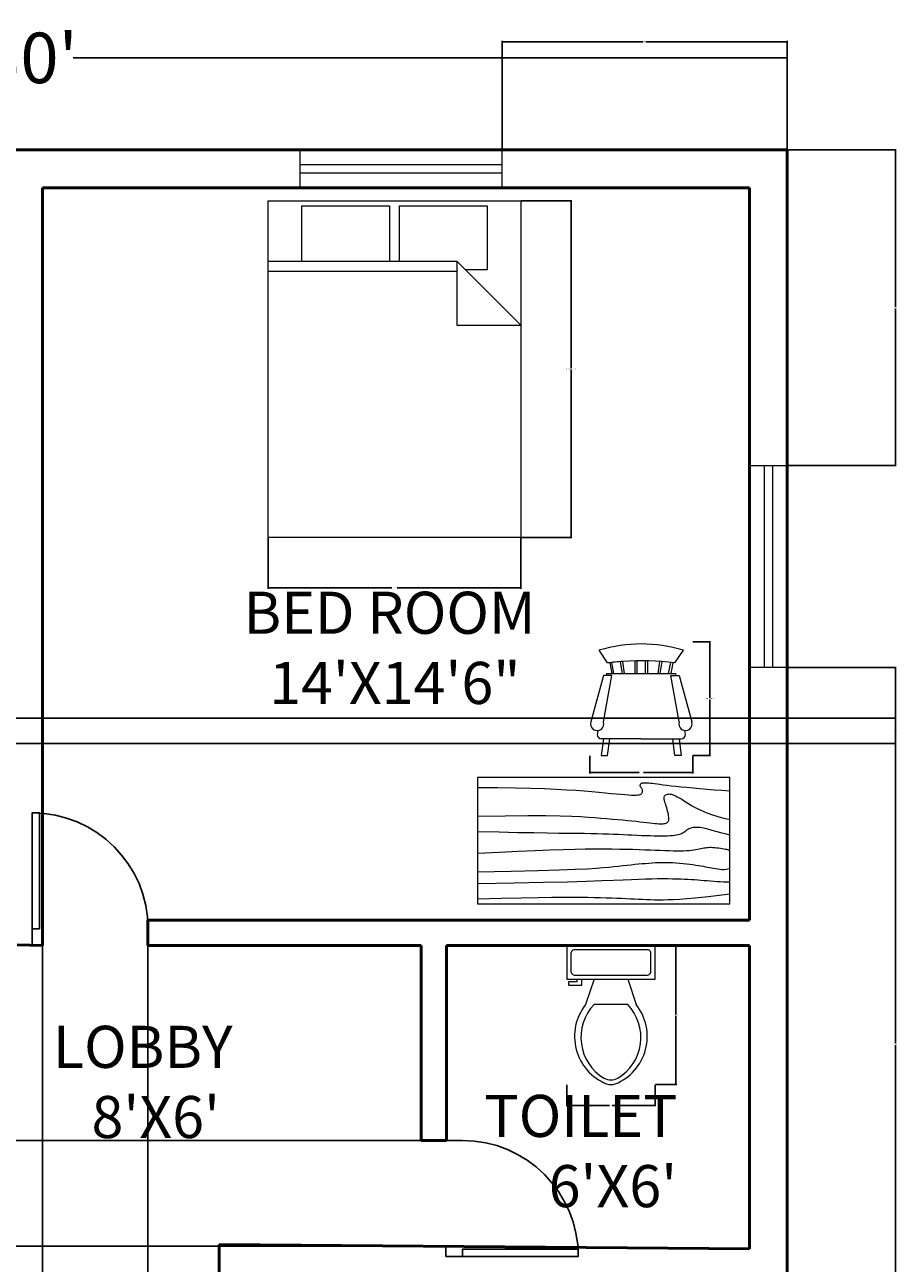
# Model space of a CAD drawing. Units: inches. Extents: x 471 to 898, y -3 to 533.
# Tile 3 of 3: x 691 to 898, y 239 to 533. Entities that reach past the tile are written whole.
import ezdxf

# ---------------------------------------------------------------- set-up
doc = ezdxf.new("R2010")
doc.units = ezdxf.units.IN
doc.header["$MEASUREMENT"] = 0
for name, color, linetype, lineweight in [('A-ANNO-DIMS', 2, 'Continuous', 18), ('A-AREA-IDEN', 7, 'Continuous', 25), ('A-DOOR', 3, 'Continuous', 25), ('A-FLOR-FIXT', 9, 'Continuous', 18), ('A-FURN', 8, 'Continuous', 18), ('A-GLAZ', 4, 'Continuous', 18), ('A-WALL', 7, 'Continuous', 50)]:
    doc.layers.add(name, color=color, linetype=linetype, lineweight=lineweight)
doc.styles.get("Standard").update_dxf_attribs({"font": 'arial.ttf'})
doc.dimstyles.get("Standard").update_dxf_attribs({"dimtxt": 0.18, "dimasz": 0.18, "dimexe": 0.18, "dimexo": 0.0625, "dimgap": 0.09, "dimtad": 0, "dimtih": 1, "dimtoh": 1, "dimdec": 1, "dimzin": 0, "dimdsep": 46, "dimlunit": 4, "dimtxsty": 'Standard', "dimcen": 0.09, "dimadec": 0, "dimazin": 0, "dimtfac": 1, "dimtdec": 1, "dimtofl": 0, "dimtmove": 0, "dimatfit": 3, "dimfxl": 1, "dimtolj": 1, "dimtzin": 0, "dimarcsym": 0})

# ---------------------------------------------------------------- blocks, each defined once
blk = doc.blocks.new('Bed - Queen')
for p, q in [((0, -80.00003), (0, 0)), ((0, 0), (59.99999, 0)), ((59.99999, 0), (59.99999, -80.00003)), ((7.99999, -1.2), (28.79998, -1.2)), ((7.99999, -14.4), (7.99999, -1.2)), ((28.79998, -1.2), (28.79998, -14.4)), ((31.19999, -1.2), (51.99999, -1.2)), ((31.19999, -14.4), (31.19999, -1.2)), ((51.99999, -1.2), (51.99999, -16.4)), ((0, -14.4), (44.8, -14.4)), ((59.99999, -29.6), (44.8, -14.4)), ((44.8, -14.4), (44.8, -29.6)), ((44.8, -16.8), (0, -16.8)), ((51.99999, -16.4), (46.79936, -16.4)), ((44.8, -29.6), (59.99999, -29.6)), ((59.99999, -80.00003), (0, -80.00003))]:
    blk.add_line(p, q)
blk = doc.blocks.new('Table - Rectangular Woodgrain 60 x 30 in.')
for p, q in [((0, 0), (0, -30)), ((60, 0), (0, 0)), ((60, -30), (60, 0)), ((0, -30), (60, -30))]:
    blk.add_line(p, q)
for points in [[(0, -2.4), (4.8155, -2.418), (9.0302, -2.4688), (12.709, -2.5477), (15.9167, -2.65), (18.7181, -2.7711), (21.1781, -2.9063), (23.3616, -3.0508), (25.3333, -3.2), (27.1477, -3.3495), (28.8172, -3.4958), (30.3437, -3.636), (31.7291, -3.7667), (32.9756, -3.8849), (34.0849, -3.9875), (35.059, -4.0714), (35.9, -4.1334), (36.6114, -4.1711), (37.2041, -4.1854), (37.6906, -4.1779), (38.0833, -4.15), (38.3948, -4.1034), (38.6375, -4.0396), (38.8239, -3.9602), (38.9666, -3.8667), (39.0764, -3.7608), (39.1573, -3.6448), (39.2116, -3.521), (39.2416, -3.3917), (39.2498, -3.2593), (39.2385, -3.1261), (39.21, -2.9944), (39.1666, -2.8667), (39.111, -2.7447), (39.0468, -2.6281), (38.978, -2.5163), (38.9083, -2.4083), (38.8418, -2.3035), (38.7823, -2.201), (38.7337, -2.1001), (38.7, -2), (38.6844, -1.9003), (38.6875, -1.8021), (38.7094, -1.707), (38.75, -1.6167), (38.8094, -1.5326), (38.8875, -1.4563), (38.9844, -1.3893), (39.1, -1.3333), (39.2351, -1.2896), (39.3937, -1.2583), (39.5804, -1.2396), (39.8, -1.2333), (40.057, -1.2396), (40.3562, -1.2583), (40.7023, -1.2896), (41.1, -1.3333), (41.5547, -1.3895), (42.0755, -1.4573), (42.6721, -1.5361), (43.3542, -1.625), (44.1316, -1.7233), (45.014, -1.8302), (46.0114, -1.9449), (47.1333, -2.0667), (48.3862, -2.1947), (49.7625, -2.3281), (51.2513, -2.4663), (52.8416, -2.6083), (54.5226, -2.7535), (56.2833, -2.9011), (58.1127, -3.0501), (60, -3.2)], [(0, -9.2), (6.5759, -9.0858), (11.9385, -9.0365), (16.2527, -9.0418), (19.6833, -9.0917), (22.3952, -9.1759), (24.5531, -9.2844), (26.322, -9.4069), (27.8666, -9.5333), (29.3241, -9.6553), (30.7203, -9.7719), (32.0532, -9.8837), (33.3208, -9.9917), (34.5213, -10.0965), (35.6526, -10.199), (36.7128, -10.2999), (37.7, -10.4), (38.6129, -10.4996), (39.4531, -10.5969), (40.223, -10.6895), (40.925, -10.775), (41.5613, -10.8512), (42.1344, -10.9156), (42.6465, -10.966), (43.1, -11), (43.4976, -11.0158), (43.8437, -11.0136), (44.143, -10.9942), (44.4, -10.9583), (44.6195, -10.9069), (44.8062, -10.8406), (44.9648, -10.7603), (45.1, -10.6667), (45.2155, -10.5598), (45.3114, -10.4365), (45.3871, -10.2929), (45.4416, -10.125), (45.4743, -9.929), (45.4844, -9.7011), (45.4709, -9.4371), (45.4333, -9.1333), (45.3716, -8.7883), (45.2896, -8.4104), (45.1919, -8.0107), (45.0833, -7.6), (44.9685, -7.1893), (44.8521, -6.7896), (44.7388, -6.4117), (44.6333, -6.0667), (44.54, -5.7628), (44.4614, -5.4979), (44.4001, -5.2675), (44.3583, -5.0667), (44.3384, -4.8909), (44.3427, -4.7354), (44.3736, -4.5956), (44.4333, -4.4667), (44.5236, -4.3453), (44.6427, -4.2333), (44.7884, -4.1339), (44.9583, -4.05), (45.1501, -3.9849), (45.3614, -3.9417), (45.59, -3.9234), (45.8333, -3.9333), (46.0915, -3.9749), (46.3734, -4.0531), (46.6906, -4.1736), (47.0542, -4.3417), (47.4756, -4.5629), (47.9661, -4.8427), (48.5372, -5.1866), (49.2, -5.6), (49.9676, -6.0844), (50.8594, -6.625), (51.8965, -7.2031), (53.1, -7.8), (54.491, -8.3969), (56.0906, -8.975), (57.9199, -9.5156), (60, -10)], [(0, -12.8), (5.1847, -12.9322), (9.6213, -13.0323), (13.3963, -13.1059), (16.5958, -13.1583), (19.3063, -13.1952), (21.614, -13.2219), (23.6054, -13.2439), (25.3666, -13.2667), (26.9728, -13.2947), (28.4531, -13.3281), (29.8256, -13.3663), (31.1083, -13.4083), (32.3191, -13.4535), (33.476, -13.501), (34.597, -13.5501), (35.7, -13.6), (36.7984, -13.6497), (37.8875, -13.6979), (38.9578, -13.743), (40, -13.7833), (41.0047, -13.8174), (41.9625, -13.8438), (42.864, -13.8607), (43.7, -13.8667), (44.4631, -13.8604), (45.1552, -13.8417), (45.7801, -13.8104), (46.3416, -13.7667), (46.8439, -13.7104), (47.2906, -13.6417), (47.6858, -13.5604), (48.0333, -13.4667), (48.3375, -13.3608), (48.6042, -13.2448), (48.8396, -13.121), (49.05, -12.9917), (49.2417, -12.8593), (49.4208, -12.7261), (49.5937, -12.5944), (49.7667, -12.4667), (49.9452, -12.3451), (50.1323, -12.2313), (50.3303, -12.1268), (50.5416, -12.0333), (50.7686, -11.9524), (51.0135, -11.8854), (51.2788, -11.8341), (51.5666, -11.8), (51.8785, -11.7843), (52.2116, -11.7865), (52.562, -11.8059), (52.926, -11.8417), (53.2998, -11.8931), (53.6795, -11.9594), (54.0614, -12.0397), (54.4416, -12.1333), (54.8223, -12.2401), (55.2293, -12.3625), (55.6942, -12.5037), (56.2489, -12.6667), (56.9251, -12.8547), (57.7545, -13.0708), (58.7689, -13.3182), (60, -13.6)], [(0, -18), (5.124, -17.7273), (9.6609, -17.5057), (13.6705, -17.3303), (17.2125, -17.1958), (20.3467, -17.0973), (23.1328, -17.0297), (25.6307, -16.9878), (27.9, -16.9667), (29.9928, -16.9617), (31.9302, -16.9703), (33.7254, -16.9907), (35.3917, -17.0208), (36.9423, -17.0588), (38.3906, -17.1026), (39.7499, -17.1503), (41.0333, -17.2), (42.2519, -17.2496), (43.4073, -17.2969), (44.4986, -17.3395), (45.525, -17.375), (46.4858, -17.4012), (47.3802, -17.4156), (48.2074, -17.416), (48.9667, -17.4), (49.6583, -17.3662), (50.2872, -17.3167), (50.8595, -17.2547), (51.3812, -17.1833), (51.8584, -17.1057), (52.2971, -17.025), (52.7034, -16.9443), (53.0833, -16.8667), (53.443, -16.7951), (53.789, -16.7313), (54.128, -16.6768), (54.4666, -16.6334), (54.8115, -16.6024), (55.1693, -16.5854), (55.5465, -16.5841), (55.95, -16.6), (56.3828, -16.6337), (56.8346, -16.6823), (57.2915, -16.7418), (57.7396, -16.8084), (58.165, -16.878), (58.5539, -16.9469), (58.8924, -17.0111), (59.1666, -17.0667), (59.3679, -17.1107), (59.5078, -17.1438), (59.6032, -17.1675), (59.6708, -17.1833), (59.7275, -17.193), (59.7901, -17.1979), (59.8753, -17.1998), (60, -17.2)], [(0, -22.4), (8.0098, -22.2501), (14.4094, -22.1011), (19.4168, -21.9535), (23.25, -21.8083), (26.1269, -21.6663), (28.2656, -21.5281), (29.884, -21.3947), (31.2, -21.2667), (32.3967, -21.1448), (33.5172, -21.0292), (34.5697, -20.9198), (35.5625, -20.8167), (36.5037, -20.7198), (37.4015, -20.6292), (38.2642, -20.5448), (39.1, -20.4667), (39.9164, -20.3951), (40.7187, -20.3313), (41.5117, -20.2768), (42.3, -20.2333), (43.0883, -20.2024), (43.8812, -20.1854), (44.6836, -20.1841), (45.5, -20.2), (46.3328, -20.234), (47.1747, -20.2844), (48.0163, -20.3488), (48.8479, -20.425), (49.66, -20.5106), (50.4429, -20.6031), (51.1872, -20.7004), (51.8833, -20.8), (52.5246, -20.8999), (53.1166, -20.9995), (53.6681, -21.0983), (54.1875, -21.1958), (54.6834, -21.2919), (55.1646, -21.3859), (55.6394, -21.4777), (56.1167, -21.5667), (56.6028, -21.6515), (57.0961, -21.7266), (57.5929, -21.7852), (58.0896, -21.8208), (58.5823, -21.8268), (59.0674, -21.7964), (59.5412, -21.723), (60, -21.6)], [(0, -25.2), (8.6355, -25.0504), (15.7026, -24.9031), (21.4049, -24.7606), (25.9458, -24.625), (29.529, -24.4988), (32.3578, -24.3844), (34.6359, -24.284), (36.5667, -24.2), (38.3213, -24.1341), (39.9417, -24.0854), (41.437, -24.0523), (42.8167, -24.0333), (44.0901, -24.0268), (45.2667, -24.0313), (46.3557, -24.0451), (47.3667, -24.0667), (48.309, -24.0947), (49.1928, -24.1287), (50.0284, -24.168), (50.826, -24.2125), (51.5959, -24.2617), (52.3483, -24.3151), (53.0935, -24.3725), (53.8417, -24.4334), (54.6009, -24.497), (55.3699, -24.561), (56.1454, -24.6226), (56.9239, -24.6792), (57.7021, -24.7279), (58.4764, -24.7662), (59.2435, -24.7911), (60, -24.8)], [(0, -28.8), (5.6867, -28.6681), (10.45, -28.5698), (14.407, -28.5012), (17.675, -28.4584), (20.3711, -28.4374), (22.6125, -28.4344), (24.5164, -28.4455), (26.2, -28.4667), (27.762, -28.4947), (29.2276, -28.5281), (30.6033, -28.5663), (31.8958, -28.6084), (33.1118, -28.6535), (34.2578, -28.7011), (35.3405, -28.7501), (36.3666, -28.8), (37.3443, -28.8497), (38.288, -28.8974), (39.2137, -28.9412), (40.1375, -28.9792), (41.0753, -29.0093), (42.0432, -29.0297), (43.0572, -29.0384), (44.1333, -29.0333), (45.2936, -29.0114), (46.5843, -28.9641), (48.0579, -28.8816), (49.7666, -28.7542), (51.7629, -28.5721), (54.0989, -28.3255), (56.8272, -28.0048), (60, -27.6)]]:
    blk.add_lwpolyline(points)
blk = doc.blocks.new('Chair - Rocking')
for p, q in [((-8, -4.5), (-10, -1.5)), ((8, -4.5), (10, -1.5)), ((-7.5, -4.5), (-7, -7)), ((-6.5, -7), (-7.02225, -4.43)), ((-4.5, -7), (-4.96674, -4.19951)), ((-4, -7), (-4.40532, -4.16272)), ((-1.5, -4.05012), (-1.5, -7)), ((-1, -7), (-1, -4.05012)), ((1, -7), (1, -4.04655)), ((1.5, -4.05012), (1.5, -7)), ((4, -7), (4.40187, -4.18694)), ((4.5, -7), (4.96761, -4.19437)), ((6.5, -7), (7, -4.4057)), ((7.5, -4.5), (7, -7)), ((-9, -7.5), (-12, -18.49999)), ((-7, -7.5), (-9, -7.5)), ((-9, -18.49999), (-7, -7.5)), ((-8.23428, -6.99939), (-8.3093, -7.47958)), ((-8.23041, -7), (8.23915, -7)), ((7, -7.5), (9, -7.5)), ((9, -18.49999), (7, -7.5)), ((8.31071, -7.48854), (8.23449, -7.00073)), ((9, -7.5), (12, -18.49999)), ((10.5, -21.49999), (10.3575, -20.58798)), ((-10.36644, -20.64523), (-10.5, -21.49999)), ((-9, -22.49999), (-9.5, -26.49999)), ((0, -22.49999), (-9.5, -22.49999)), ((-8, -26.49999), (-7.5, -22.49999)), ((0, -22.49999), (9.5, -22.49999)), ((8, -26.49999), (7.5, -22.49999)), ((9, -22.49999), (9.5, -26.49999)), ((-9.5, -26.49999), (-8, -26.49999)), ((9.5, -26.49999), (8, -26.49999))]:
    blk.add_line(p, q)
for centre, radius, start, end in [((0, -34.08333), 34.08333, 72.93847, 107.0615), ((0, -68.25004), 64.25, 93.92211, 97.15267), ((0, -68.25004), 64.25, 82.84733, 93.92211), ((-10.5, -18.99999), 1.58114, 161.5651, 18.43495), ((10.5, -18.99999), 1.58114, 161.5651, 18.43495), ((-9.5, -21.49999), 1, 180, 270), ((9.5, -21.49999), 1, 270, 0)]:
    blk.add_arc(centre, radius, start, end)
blk = doc.blocks.new('*U8')
for p, q in [((0, 0), (0, -100)), ((700, 0), (700, -100))]:
    blk.add_line(p, q)
blk.add_lwpolyline([(0, 0), (0, 700), (43.75, 700), (43.75, 0)], close=True)
blk.add_arc((0, 0), 700, 0, 90)
blk = doc.blocks.new('Toilet - top')
for p, q in [((9.5, -6), (9.5, -2)), ((-10, -8.5), (-8, -8.5)), ((-10, -9.5), (-10, -8.5)), ((-8, -8.5), (-8, -8)), ((-7, -8), (-7, -9.5)), ((-4, -8), (-6, -14)), ((4, -8), (6, -14)), ((-7, -9.5), (-10, -9.5)), ((4, -14), (-4, -14))]:
    blk.add_line(p, q)
blk.add_lwpolyline([(10.5, -8), (10.5, 0), (-10.5, 0), (-10.5, -8)], close=True)
for points in [[(-9.5, -2), (-9.5, -6)], [(8.5, -1), (-8.5, -1)], [(-8.5, -7), (8.5, -7)]]:
    blk.add_lwpolyline(points)
for centre, radius, start, end in [((-8.62, -1.88), 0.884, 81.8699, 188.1301), ((8.62, -1.88), 0.884, 351.8699, 98.1301), ((-8.62, -6.12), 0.884, 171.8699, 278.1301), ((8.62, -6.12), 0.884, 261.8699, 8.1301), ((3.52, -21.58), 12.17, 141.4691, 247.9714), ((4.2, -21.82), 11.33, 136.3677, 238.9468), ((-3.52, -21.58), 12.17, 292.0284, 38.5307), ((-4.2, -21.82), 11.33, 301.053, 43.6321), ((0, -27.88), 4, 245.7318, 294.2682), ((0, -29), 4, 254.8605, 285.1395)]:
    blk.add_arc(centre, radius, start, end)
blk = doc.blocks.new('*D12')
at = {"layer": 'A-ANNO-DIMS', "color": 0, "lineweight": -2, "transparency": 16777216}
for p, q in [((512.23, 503.14), (512.23, 525.11)), ((512.41, 524.93), (681.96, 524.93)), ((872.05, 524.93), (702.5, 524.93)), ((872.23, 503.14), (872.23, 525.11))]:
    blk.add_line(p, q, dxfattribs=at)
at = {"layer": 'A-ANNO-DIMS', "color": 0, "transparency": 16777216}
for points in [[(512.41, 524.96), (512.41, 524.9), (512.23, 524.93)], [(872.05, 524.96), (872.05, 524.9), (872.23, 524.93)]]:
    blk.add_solid(points, dxfattribs=at)
at = {"layer": 'Defpoints', "color": 0, "transparency": 16777216}
for p in [(872.23, 524.93), (512.23, 503.07), (872.23, 503.07)]:
    blk.add_point(p, dxfattribs=at)
at = {"layer": 'A-ANNO-DIMS', "color": 0, "transparency": 16777216, "insert": (692.23, 524.93), "char_height": 12, "attachment_point": 5}
blk.add_mtext("\\A1;30'", dxfattribs=at)
blk = doc.blocks.new('WIN-48X9')
for p, q in [((0, 48), (9, 48)), ((0, 0), (0, 48)), ((3.5, 48), (3.5, 0)), ((5.5, 48), (5.5, 0)), ((9, 48), (9, 0)), ((9, 0), (0, 0))]:
    blk.add_line(p, q)
blk = doc.blocks.new('*D17')
at = {"layer": 'A-ANNO-DIMS', "color": 0, "lineweight": -2, "transparency": 16777216}
for p, q in [((808.96, 491.01), (821.07, 491.01)), ((820.89, 490.83), (820.89, 451.2)), ((820.89, 411.19), (820.89, 450.82)), ((808.96, 411.01), (821.07, 411.01))]:
    blk.add_line(p, q, dxfattribs=at)
at = {"layer": 'A-ANNO-DIMS', "color": 0, "transparency": 16777216}
for points in [[(820.86, 490.83), (820.92, 490.83), (820.89, 491.01)], [(820.86, 411.19), (820.92, 411.19), (820.89, 411.01)]]:
    blk.add_solid(points, dxfattribs=at)
at = {"layer": 'Defpoints', "color": 0, "transparency": 16777216}
for p in [(808.89, 491.01), (820.89, 491.01), (808.89, 411.01)]:
    blk.add_point(p, dxfattribs=at)
at = {"layer": 'A-ANNO-DIMS', "color": 0, "transparency": 16777216, "insert": (820.89, 451.01), "char_height": 0.18, "attachment_point": 5}
blk.add_mtext('\\A1;QUEEN BED 6\'-8" TYP.', dxfattribs=at)
blk = doc.blocks.new('*D18')
at = {"layer": 'A-ANNO-DIMS', "color": 0, "lineweight": -2, "transparency": 16777216}
for p, q in [((748.89, 410.95), (748.89, 398.83)), ((808.89, 410.95), (808.89, 398.83)), ((749.07, 399.01), (778.25, 399.01)), ((808.71, 399.01), (779.53, 399.01))]:
    blk.add_line(p, q, dxfattribs=at)
at = {"layer": 'A-ANNO-DIMS', "color": 0, "transparency": 16777216}
for points in [[(749.07, 399.04), (749.07, 398.98), (748.89, 399.01)], [(808.71, 399.04), (808.71, 398.98), (808.89, 399.01)]]:
    blk.add_solid(points, dxfattribs=at)
at = {"layer": 'Defpoints', "color": 0, "transparency": 16777216}
for p in [(748.89, 411.01), (808.89, 411.01), (808.89, 399.01)]:
    blk.add_point(p, dxfattribs=at)
at = {"layer": 'A-ANNO-DIMS', "color": 0, "transparency": 16777216, "insert": (778.89, 399.01), "char_height": 0.18, "attachment_point": 5}
blk.add_mtext('\\A1;5\'-0" TYP.', dxfattribs=at)
blk = doc.blocks.new('*D27')
at = {"layer": 'A-ANNO-DIMS', "color": 0, "lineweight": -2, "transparency": 16777216}
for p, q in [((849.82, 386.21), (853.99, 386.21)), ((853.81, 386.03), (853.81, 372.89)), ((853.81, 359.39), (853.81, 372.53)), ((849.82, 359.21), (853.99, 359.21))]:
    blk.add_line(p, q, dxfattribs=at)
at = {"layer": 'A-ANNO-DIMS', "color": 0, "transparency": 16777216}
for points in [[(853.78, 386.03), (853.84, 386.03), (853.81, 386.21)], [(853.78, 359.39), (853.84, 359.39), (853.81, 359.21)]]:
    blk.add_solid(points, dxfattribs=at)
at = {"layer": 'Defpoints', "color": 0, "transparency": 16777216}
for p in [(849.76, 386.21), (853.81, 386.21), (849.76, 359.21)]:
    blk.add_point(p, dxfattribs=at)
at = {"layer": 'A-ANNO-DIMS', "color": 0, "transparency": 16777216, "insert": (853.81, 372.71), "char_height": 0.18, "attachment_point": 5}
blk.add_mtext('\\A1;ROCKING CHAIR 2\'-3"', dxfattribs=at)
blk = doc.blocks.new('*D28')
at = {"layer": 'A-ANNO-DIMS', "color": 0, "lineweight": -2, "transparency": 16777216}
for p, q in [((825.32, 359.15), (825.32, 354.98)), ((849.76, 359.15), (849.76, 354.98)), ((825.5, 355.16), (837, 355.16)), ((849.58, 355.16), (838.08, 355.16))]:
    blk.add_line(p, q, dxfattribs=at)
at = {"layer": 'A-ANNO-DIMS', "color": 0, "transparency": 16777216}
for points in [[(825.5, 355.19), (825.5, 355.13), (825.32, 355.16)], [(849.58, 355.19), (849.58, 355.13), (849.76, 355.16)]]:
    blk.add_solid(points, dxfattribs=at)
at = {"layer": 'Defpoints', "color": 0, "transparency": 16777216}
for p in [(825.32, 359.21), (849.76, 359.21), (849.76, 355.16)]:
    blk.add_point(p, dxfattribs=at)
at = {"layer": 'A-ANNO-DIMS', "color": 0, "transparency": 16777216, "insert": (837.54, 355.16), "char_height": 0.18, "attachment_point": 5}
blk.add_mtext('\\A1;2\'-0 1/2"', dxfattribs=at)
blk = doc.blocks.new('*D31')
at = {"layer": 'A-ANNO-DIMS', "color": 0, "lineweight": -2, "transparency": 16777216}
for p, q in [((840.89, 314.07), (845.96, 314.07)), ((845.78, 313.89), (845.78, 297.73)), ((845.78, 281.21), (845.78, 297.37)), ((840.89, 281.03), (845.96, 281.03))]:
    blk.add_line(p, q, dxfattribs=at)
at = {"layer": 'A-ANNO-DIMS', "color": 0, "transparency": 16777216}
for points in [[(845.75, 313.89), (845.81, 313.89), (845.78, 314.07)], [(845.75, 281.21), (845.81, 281.21), (845.78, 281.03)]]:
    blk.add_solid(points, dxfattribs=at)
at = {"layer": 'Defpoints', "color": 0, "transparency": 16777216}
for p in [(840.82, 314.07), (845.78, 314.07), (840.82, 281.03)]:
    blk.add_point(p, dxfattribs=at)
at = {"layer": 'A-ANNO-DIMS', "color": 0, "transparency": 16777216, "insert": (845.78, 297.55), "char_height": 0.18, "attachment_point": 5}
blk.add_mtext('\\A1;WC 2\'-9"', dxfattribs=at)
blk = doc.blocks.new('*D32')
at = {"layer": 'A-ANNO-DIMS', "color": 0, "lineweight": -2, "transparency": 16777216}
for p, q in [((819.82, 280.97), (819.82, 275.89)), ((840.82, 280.97), (840.82, 275.89)), ((820, 276.07), (830, 276.07)), ((840.64, 276.07), (830.64, 276.07))]:
    blk.add_line(p, q, dxfattribs=at)
at = {"layer": 'A-ANNO-DIMS', "color": 0, "transparency": 16777216}
for points in [[(820, 276.1), (820, 276.04), (819.82, 276.07)], [(840.64, 276.1), (840.64, 276.04), (840.82, 276.07)]]:
    blk.add_solid(points, dxfattribs=at)
at = {"layer": 'Defpoints', "color": 0, "transparency": 16777216}
for p in [(819.82, 281.03), (840.82, 281.03), (840.82, 276.07)]:
    blk.add_point(p, dxfattribs=at)
at = {"layer": 'A-ANNO-DIMS', "color": 0, "transparency": 16777216, "insert": (830.32, 276.07), "char_height": 0.18, "attachment_point": 5}
blk.add_mtext('\\A1;1\'-9"', dxfattribs=at)
blk = doc.blocks.new('*D38')
at = {"layer": 'A-ANNO-DIMS', "color": 0, "lineweight": -2, "transparency": 16777216}
for p, q in [((804.44, 503.14), (804.44, 528.95)), ((804.62, 528.77), (838, 528.77)), ((872.05, 528.77), (838.66, 528.77)), ((872.23, 503.14), (872.23, 528.95))]:
    blk.add_line(p, q, dxfattribs=at)
at = {"layer": 'A-ANNO-DIMS', "color": 0, "transparency": 16777216}
for points in [[(804.62, 528.8), (804.62, 528.74), (804.44, 528.77)], [(872.05, 528.8), (872.05, 528.74), (872.23, 528.77)]]:
    blk.add_solid(points, dxfattribs=at)
at = {"layer": 'Defpoints', "color": 0, "transparency": 16777216}
for p in [(872.23, 528.77), (804.44, 503.07), (872.23, 503.07)]:
    blk.add_point(p, dxfattribs=at)
at = {"layer": 'A-ANNO-DIMS', "color": 0, "transparency": 16777216, "insert": (838.33, 528.77), "char_height": 0.18, "attachment_point": 5}
blk.add_mtext('\\A1;5\'-8"', dxfattribs=at)
blk = doc.blocks.new('*D39')
at = {"layer": 'A-ANNO-DIMS', "color": 0, "lineweight": -2, "transparency": 16777216}
for p, q in [((872.29, 503.07), (898.15, 503.07)), ((897.97, 502.89), (897.97, 465.76)), ((897.97, 428.27), (897.97, 465.4)), ((872.29, 428.09), (898.15, 428.09))]:
    blk.add_line(p, q, dxfattribs=at)
at = {"layer": 'A-ANNO-DIMS', "color": 0, "transparency": 16777216}
for points in [[(897.94, 502.89), (898, 502.89), (897.97, 503.07)], [(897.94, 428.27), (898, 428.27), (897.97, 428.09)]]:
    blk.add_solid(points, dxfattribs=at)
at = {"layer": 'Defpoints', "color": 0, "transparency": 16777216}
for p in [(872.23, 503.07), (872.23, 428.09), (897.97, 428.09)]:
    blk.add_point(p, dxfattribs=at)
at = {"layer": 'A-ANNO-DIMS', "color": 0, "transparency": 16777216, "insert": (897.97, 465.58), "char_height": 0.18, "attachment_point": 5}
blk.add_mtext('\\A1;6\'-3"', dxfattribs=at)
blk = doc.blocks.new('*D40')
at = {"layer": 'A-ANNO-DIMS', "color": 0, "lineweight": -2, "transparency": 16777216}
for p, q in [((872.29, 380.09), (898.15, 380.09)), ((897.97, 379.91), (897.97, 290.77)), ((897.97, 201.27), (897.97, 290.41)), ((872.33, 201.09), (898.15, 201.09))]:
    blk.add_line(p, q, dxfattribs=at)
at = {"layer": 'A-ANNO-DIMS', "color": 0, "transparency": 16777216}
for points in [[(897.94, 379.91), (898, 379.91), (897.97, 380.09)], [(897.94, 201.27), (898, 201.27), (897.97, 201.09)]]:
    blk.add_solid(points, dxfattribs=at)
at = {"layer": 'Defpoints', "color": 0, "transparency": 16777216}
for p in [(872.23, 380.09), (872.27, 201.09), (897.97, 201.09)]:
    blk.add_point(p, dxfattribs=at)
at = {"layer": 'A-ANNO-DIMS', "color": 0, "transparency": 16777216, "insert": (897.97, 290.59), "char_height": 0.18, "attachment_point": 5}
blk.add_mtext('\\A1;14\'-11"', dxfattribs=at)
blk = doc.blocks.new('*D45')
at = {"layer": 'A-ANNO-DIMS', "color": 0, "lineweight": -2, "transparency": 16777216}
for p, q in [((612.9, 368.07), (898.15, 368.07)), ((897.97, 367.89), (897.97, 365.26)), ((897.97, 362.25), (897.97, 364.89)), ((612.9, 362.07), (898.15, 362.07))]:
    blk.add_line(p, q, dxfattribs=at)
at = {"layer": 'A-ANNO-DIMS', "color": 0, "transparency": 16777216}
for points in [[(897.94, 367.89), (898, 367.89), (897.97, 368.07)], [(897.94, 362.25), (898, 362.25), (897.97, 362.07)]]:
    blk.add_solid(points, dxfattribs=at)
at = {"layer": 'Defpoints', "color": 0, "transparency": 16777216}
for p in [(612.83, 368.07), (897.97, 368.07), (612.83, 362.07)]:
    blk.add_point(p, dxfattribs=at)
at = {"layer": 'A-ANNO-DIMS', "color": 0, "transparency": 16777216, "insert": (897.97, 365.07), "char_height": 0.18, "attachment_point": 5}
blk.add_mtext('\\A1;0\'-6"', dxfattribs=at)
blk = doc.blocks.new('*D48')
at = {"layer": 'A-ANNO-DIMS', "color": 0, "lineweight": -2, "transparency": 16777216}
for p, q in [((695.23, 314.01), (695.23, -2.81)), ((720.23, 314.01), (720.23, -2.81)), ((695.41, -2.63), (707.4, -2.63)), ((720.05, -2.63), (708.06, -2.63))]:
    blk.add_line(p, q, dxfattribs=at)
at = {"layer": 'A-ANNO-DIMS', "color": 0, "transparency": 16777216}
for points in [[(695.41, -2.6), (695.41, -2.66), (695.23, -2.63)], [(720.05, -2.6), (720.05, -2.66), (720.23, -2.63)]]:
    blk.add_solid(points, dxfattribs=at)
at = {"layer": 'Defpoints', "color": 0, "transparency": 16777216}
for p in [(695.23, 314.07), (720.23, 314.07), (720.23, -2.63)]:
    blk.add_point(p, dxfattribs=at)
at = {"layer": 'A-ANNO-DIMS', "color": 0, "transparency": 16777216, "insert": (707.73, -2.63), "char_height": 0.18, "attachment_point": 5}
blk.add_mtext('\\A1;2\'-1"', dxfattribs=at)
blk = doc.blocks.new('*D50')
at = {"layer": 'A-ANNO-DIMS', "color": 0, "lineweight": -2, "transparency": 16777216}
for p, q in [((785.17, 267.78), (486.35, 267.78)), ((486.53, 267.6), (486.53, 255.39)), ((486.53, 242.81), (486.53, 255.03)), ((791.03, 242.63), (486.35, 242.63))]:
    blk.add_line(p, q, dxfattribs=at)
at = {"layer": 'A-ANNO-DIMS', "color": 0, "transparency": 16777216}
for points in [[(486.5, 267.6), (486.56, 267.6), (486.53, 267.78)], [(486.5, 242.81), (486.56, 242.81), (486.53, 242.63)]]:
    blk.add_solid(points, dxfattribs=at)
at = {"layer": 'Defpoints', "color": 0, "transparency": 16777216}
for p in [(486.53, 267.78), (785.23, 267.78), (791.1, 242.63)]:
    blk.add_point(p, dxfattribs=at)
at = {"layer": 'A-ANNO-DIMS', "color": 0, "transparency": 16777216, "insert": (486.53, 255.21), "char_height": 0.18, "attachment_point": 5}
blk.add_mtext('\\A1;2\'-1"', dxfattribs=at)

msp = doc.modelspace()

# ---------------------------------------------------------------- linework, layer by layer
at = {"layer": 'A-DOOR'}
for p, q in [((692.76, 314.12), (695.23, 314.07)), ((791.08, 240.22), (791.1, 242.63))]:
    msp.add_line(p, q, dxfattribs=at)
at = {"layer": 'A-WALL'}
for p, q in [((512.23, 503.07), (872.23, 503.07)), ((872.23, 23.07), (872.23, 503.07)), ((695.23, 494.07), (695.23, 368.07)), ((695.23, 494.07), (695.23, 320.07)), ((695.23, 494.07), (863.23, 494.07)), ((863.23, 320.07), (863.23, 494.07)), ((695.23, 362.07), (695.23, 314.07)), ((695.23, 320.07), (695.23, 314.07)), ((720.23, 320.07), (863.23, 320.07)), ((720.23, 320.07), (720.23, 314.07)), ((695.23, 314.07), (689.23, 314.28)), ((720.23, 314.07), (785.23, 314.07)), ((785.23, 314.07), (785.23, 267.78)), ((863.23, 314.07), (791.23, 314.07)), ((791.23, 314.07), (791.23, 267.78)), ((791.23, 314.07), (863.23, 314.07)), ((863.23, 242.07), (863.23, 314.07)), ((785.23, 267.78), (791.23, 267.78)), ((863.28, 242.07), (737.24, 243.05)), ((737.24, 243.05), (737.24, 142))]:
    msp.add_line(p, q, dxfattribs=at)

# ---------------------------------------------------------------- block references
at = {"layer": 'A-DOOR', "xscale": 0.0393700787401575, "yscale": 0.0393700787401575, "zscale": 0.0393700787401575}
msp.add_blockref('*U8', (692.76, 318.05), dxfattribs=at)
at = {"layer": 'A-DOOR', "xscale": -0.0393700787401575, "yscale": 0.0393700787401575, "zscale": 0.0393700787401575, "rotation": 270}
msp.add_blockref('*U8', (795.01, 240.22), dxfattribs=at)
at = {"layer": 'A-FLOR-FIXT'}
msp.add_blockref('Toilet - top', (830.32, 314.07), dxfattribs=at)
at = {"layer": 'A-FURN'}
for name, p in [('Bed - Queen', (748.89, 491.01)), ('Chair - Rocking', (837.54, 385.71)), ('Table - Rectangular Woodgrain 60 x 30 in.', (798.61, 354))]:
    msp.add_blockref(name, p, dxfattribs=at)
at = {"layer": 'A-GLAZ', "rotation": 269.9999999999992}
msp.add_blockref('WIN-48X9', (756.43, 503.07), dxfattribs=at)
at = {"layer": 'A-GLAZ'}
msp.add_blockref('WIN-48X9', (863.23, 380.09), dxfattribs=at)

# ---------------------------------------------------------------- texts
at = {"layer": 'A-AREA-IDEN', "char_height": 10, "attachment_point": 1}
for s, insert in [('BED ROOM\\P  14\'X14\'6"', (742.99, 398.13)), ("LOBBY\\P   8'X6'", (697.69, 295.01)), ("TOILET\\P     6'X6'", (800.24, 278.6))]:
    msp.add_mtext_dynamic_manual_height_columns(s, width=80.8054, gutter_width=1, heights=[0], dxfattribs=dict(at, insert=insert))

# ---------------------------------------------------------------- dimensions: what is measured, and where the dimension line sits
at = {"layer": 'A-ANNO-DIMS'}
for base, p1, p2, override, picture, middle in [((872.23, 524.93), (512.23, 503.07), (872.23, 503.07), {"dimtxt": 12, "dimclrd": 0, "dimclre": 0, "dimclrt": 0}, '*D12', (692.23, 524.93)), ((872.23, 528.77), (804.44, 503.07), (872.23, 503.07), {"dimdec": 1, "dimlfac": 1, "dimrnd": 0, "dimzin": 1, "dimdsep": 46, "dimlunit": 4, "dimfrac": 2}, '*D38', (838.33, 528.77)), ((849.76, 355.16), (825.32, 359.21), (849.76, 359.21), {"dimdec": 1, "dimlfac": 1, "dimrnd": 0, "dimzin": 1, "dimdsep": 46, "dimlunit": 4, "dimfrac": 2}, '*D28', (837.54, 355.16)), ((720.23, -2.63), (695.23, 314.07), (720.23, 314.07), {"dimdec": 1, "dimlfac": 1, "dimrnd": 0, "dimzin": 1, "dimdsep": 46, "dimlunit": 4, "dimfrac": 2}, '*D48', (707.73, -2.63)), ((840.82, 276.07), (819.82, 281.03), (840.82, 281.03), {"dimdec": 1, "dimlfac": 1, "dimrnd": 0, "dimzin": 1, "dimdsep": 46, "dimlunit": 4, "dimfrac": 2}, '*D32', (830.32, 276.07))]:
    dim = msp.add_linear_dim(base=base, p1=p1, p2=p2, dimstyle='Standard', override=override, dxfattribs=at)
    dim.commit()
    dim.dimension.update_dxf_attribs({"geometry": picture, "text_midpoint": middle})
for base, p1, p2, picture, middle in [((897.97, 428.09), (872.23, 503.07), (872.23, 428.09), '*D39', (897.97, 465.58)), ((897.97, 201.09), (872.23, 380.09), (872.27, 201.09), '*D40', (897.97, 290.59)), ((897.97, 368.07), (612.83, 362.07), (612.83, 368.07), '*D45', (897.97, 365.07)), ((486.532, 267.7812), (791.0957, 242.6327), (785.232, 267.7812), '*D50', (486.532, 255.207))]:
    dim = msp.add_linear_dim(base=base, p1=p1, p2=p2, angle=90, dimstyle='Standard', override={"dimdec": 1, "dimlfac": 1, "dimrnd": 0, "dimzin": 1, "dimdsep": 46, "dimlunit": 4, "dimfrac": 2}, dxfattribs=at)
    dim.commit()
    dim.dimension.update_dxf_attribs({"geometry": picture, "text_midpoint": middle})
for base, p1, p2, text, picture, middle in [((820.89, 491.01), (808.89, 411.01), (808.89, 491.01), 'QUEEN BED <> TYP.', '*D17', (820.89, 451.01)), ((853.81, 386.21), (849.76, 359.21), (849.76, 386.21), 'ROCKING CHAIR <>', '*D27', (853.81, 372.71)), ((845.78, 314.07), (840.82, 281.03), (840.82, 314.07), 'WC <>', '*D31', (845.78, 297.55))]:
    dim = msp.add_linear_dim(base=base, p1=p1, p2=p2, angle=90, text=text, dimstyle='Standard', override={"dimdec": 1, "dimlfac": 1, "dimrnd": 0, "dimzin": 1, "dimdsep": 46, "dimlunit": 4, "dimfrac": 2}, dxfattribs=at)
    dim.commit()
    dim.dimension.update_dxf_attribs({"geometry": picture, "text_midpoint": middle})
dim = msp.add_linear_dim(base=(808.89, 399.01), p1=(748.89, 411.01), p2=(808.89, 411.01), text='<> TYP.', dimstyle='Standard', override={"dimdec": 1, "dimlfac": 1, "dimrnd": 0, "dimzin": 1, "dimdsep": 46, "dimlunit": 4, "dimfrac": 2}, dxfattribs=at)
dim.commit()
dim.dimension.update_dxf_attribs({"geometry": '*D18', "text_midpoint": (778.89, 399.01)})

doc.saveas('drawing.dxf')
